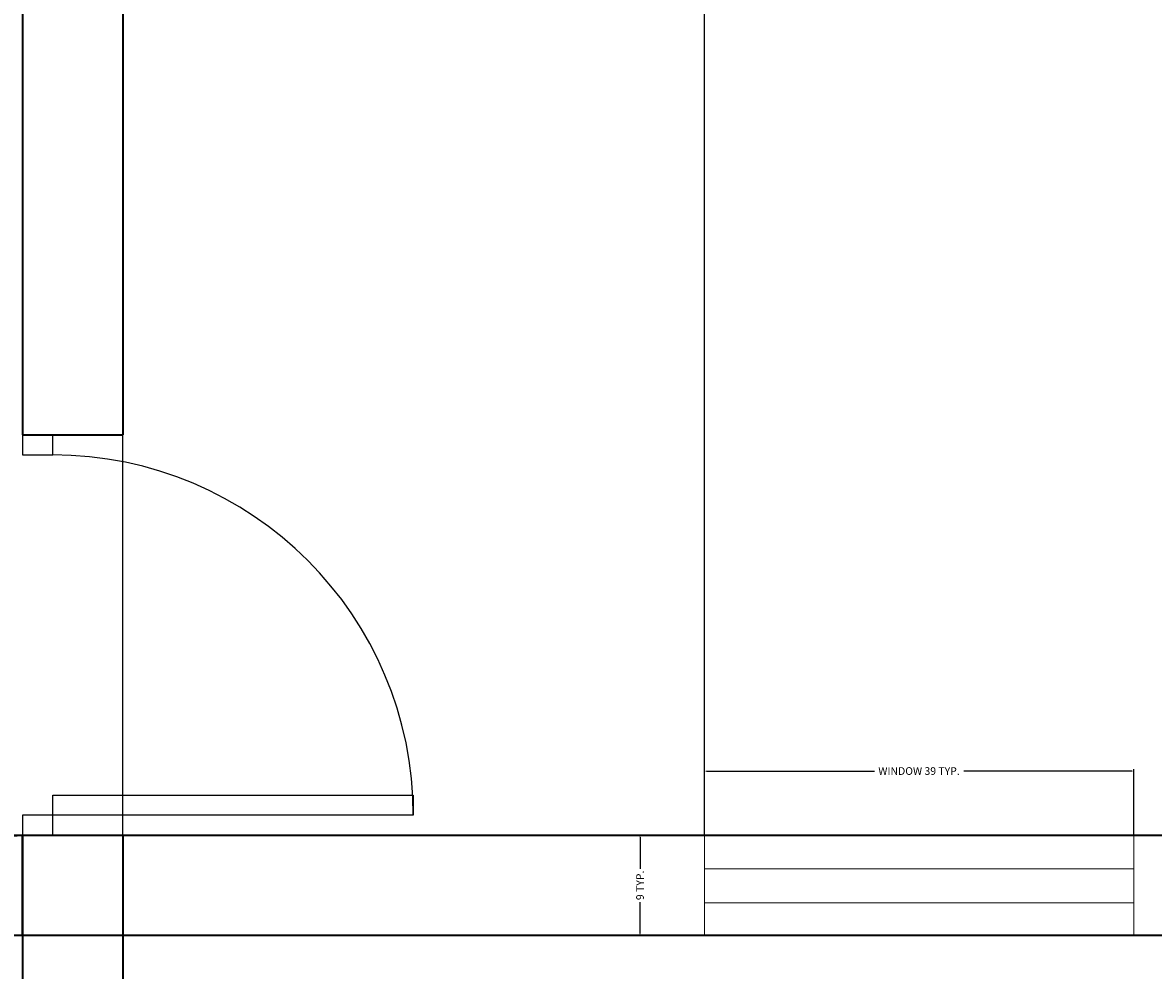
# Model space of a CAD drawing. Units: inches. Extents: x 867 to 1667, y -234 to 788.
# Tile 38 of 42: x 1395 to 1497, y 401 to 487. Entities that reach past the tile are written whole.
import ezdxf

# ---------------------------------------------------------------- set-up
doc = ezdxf.new("R2010")
doc.units = ezdxf.units.IN
doc.header["$MEASUREMENT"] = 0
for name, color, linetype, lineweight in [('A-ANNO-DIMS', 2, 'Continuous', 18), ('A-Door', 150, 'Continuous', 25), ('A-Glaz', 92, 'Continuous', 18), ('A-Wall', 7, 'Continuous', 35)]:
    doc.layers.add(name, color=color, linetype=linetype, lineweight=lineweight)
doc.layers.add('NET 01', color=8, linetype='Continuous')
doc.styles.get("Standard").update_dxf_attribs({"font": 'arial.ttf'})
doc.dimstyles.get("Standard").update_dxf_attribs({"dimtxt": 0.6875, "dimasz": 0.18, "dimexe": 0.18, "dimexo": 0.0625, "dimgap": 0.09, "dimtad": 0, "dimdec": 4, "dimzin": 0, "dimdsep": 46, "dimlunit": 4, "dimtxsty": 'Standard', "dimcen": 0.09, "dimadec": 0, "dimazin": 0, "dimtfac": 1, "dimtdec": 4, "dimtofl": 0, "dimtmove": 0, "dimatfit": 3, "dimfxl": 1, "dimtolj": 1, "dimtzin": 0, "dimarcsym": 0})

# ---------------------------------------------------------------- blocks, each defined once
blk = doc.blocks.new('A$C292B336C')
at = {"layer": 'A-Door'}
for points in [[(-0.05, 0), (-0.05, 0.9), (0, 0.9), (0, 0)], [(-0.95, 0), (-0.95, -0.075), (-0.9, -0.075), (-0.9, 0)], [(0, 0), (0, -0.075), (0.05, -0.075), (0.05, 0)]]:
    blk.add_lwpolyline(points, close=True, dxfattribs=at)
at = {"layer": 'NET 01'}
blk.add_arc((0, 0), 0.9, 90, 180, dxfattribs=at)
blk = doc.blocks.new('WIN-38_58IN')
for p, q in [((0, 9), (0, 0)), ((38.58, 0), (38.58, 9)), ((0, 6), (38.58, 6)), ((0, 2.92), (38.58, 2.92)), ((0, 0), (38.58, 0))]:
    blk.add_line(p, q)
blk = doc.blocks.new('*D13')
at = {"layer": 'A-ANNO-DIMS', "color": 0, "lineweight": -2, "transparency": 16777216}
for p, q in [((1456.15, 413.68), (1456.15, 419.58)), ((1456.33, 419.4), (1471.43, 419.4)), ((1494.56, 419.4), (1479.46, 419.4)), ((1494.74, 413.68), (1494.74, 419.58))]:
    blk.add_line(p, q, dxfattribs=at)
at = {"layer": 'A-ANNO-DIMS', "color": 0, "transparency": 16777216}
for points in [[(1456.33, 419.43), (1456.33, 419.37), (1456.15, 419.4)], [(1494.56, 419.43), (1494.56, 419.37), (1494.74, 419.4)]]:
    blk.add_solid(points, dxfattribs=at)
at = {"layer": 'Defpoints', "color": 0, "transparency": 16777216}
for p in [(1494.74, 419.4), (1456.15, 413.62), (1494.74, 413.62)]:
    blk.add_point(p, dxfattribs=at)
at = {"layer": 'A-ANNO-DIMS', "color": 0, "transparency": 16777216, "insert": (1475.44, 419.4), "char_height": 0.6875, "attachment_point": 5}
blk.add_mtext('\\A1;WINDOW 39 TYP.', dxfattribs=at)
blk = doc.blocks.new('*D14')
at = {"layer": 'A-ANNO-DIMS', "color": 0, "lineweight": -2, "transparency": 16777216}
for p, q in [((1456.09, 413.62), (1450.19, 413.62)), ((1450.37, 413.44), (1450.37, 410.61)), ((1450.37, 404.8), (1450.37, 407.62)), ((1456.09, 404.62), (1450.19, 404.62))]:
    blk.add_line(p, q, dxfattribs=at)
at = {"layer": 'A-ANNO-DIMS', "color": 0, "transparency": 16777216}
for points in [[(1450.34, 413.44), (1450.4, 413.44), (1450.37, 413.62)], [(1450.34, 404.8), (1450.4, 404.8), (1450.37, 404.62)]]:
    blk.add_solid(points, dxfattribs=at)
at = {"layer": 'Defpoints', "color": 0, "transparency": 16777216}
for p in [(1450.37, 413.62), (1456.15, 413.62), (1456.15, 404.62)]:
    blk.add_point(p, dxfattribs=at)
at = {"layer": 'A-ANNO-DIMS', "color": 0, "transparency": 16777216, "insert": (1450.37, 409.12), "char_height": 0.688, "attachment_point": 5, "rotation": 90}
blk.add_mtext('\\A1;9 TYP.', dxfattribs=at)
blk = doc.blocks.new('*D54')
at = {"layer": 'A-ANNO-DIMS', "color": 0, "lineweight": -2, "transparency": 16777216}
for p, q in [((1403.89, 413.68), (1403.89, 787.75)), ((1404.07, 787.57), (1428.77, 787.57)), ((1455.97, 787.57), (1431.27, 787.57)), ((1456.15, 413.68), (1456.15, 787.75))]:
    blk.add_line(p, q, dxfattribs=at)
at = {"layer": 'A-ANNO-DIMS', "color": 0, "transparency": 16777216}
for points in [[(1404.07, 787.6), (1404.07, 787.54), (1403.89, 787.57)], [(1455.97, 787.6), (1455.97, 787.54), (1456.15, 787.57)]]:
    blk.add_solid(points, dxfattribs=at)
at = {"layer": 'Defpoints', "color": 0, "transparency": 16777216}
for p in [(1456.15, 787.57), (1403.89, 413.62), (1456.15, 413.62)]:
    blk.add_point(p, dxfattribs=at)
at = {"layer": 'A-ANNO-DIMS', "color": 0, "transparency": 16777216, "insert": (1430.02, 787.57), "char_height": 0.688, "attachment_point": 5}
blk.add_mtext('\\A1;52.27', dxfattribs=at)

msp = doc.modelspace()

# ---------------------------------------------------------------- linework, layer by layer
at = {"layer": 'A-Wall'}
for p, q in [((1394.8866, 557.617), (1394.8866, 449.617)), ((1403.8866, 557.617), (1403.8866, 449.617)), ((1394.8866, 449.617), (1403.8866, 449.617)), ((1529.8866, 413.617), (1040.8866, 413.617)), ((1255.5362, 414.5056), (1394.8866, 404.617)), ((1394.8866, 413.617), (1256.8866, 404.617)), ((1394.8866, 413.617), (1394.8866, 136.117)), ((1394.8866, 404.617), (1394.8866, 413.617)), ((1403.8866, 413.617), (1403.8866, 136.117)), ((1559.8866, 404.617), (1040.8866, 404.617))]:
    msp.add_line(p, q, dxfattribs=at)

# ---------------------------------------------------------------- block references
at = {"layer": 'A-Door', "xscale": 36.01171521992244, "yscale": 36.01171521992244, "zscale": 36.01171521992244, "rotation": 270}
msp.add_blockref('A$C292B336C', (1397.5875, 415.4176), dxfattribs=at)
at = {"layer": 'A-Glaz'}
msp.add_blockref('WIN-38_58IN', (1456.1546, 404.617), dxfattribs=at)

# ---------------------------------------------------------------- dimensions: what is measured, and where the dimension line sits
at = {"layer": 'A-ANNO-DIMS'}
dim = msp.add_linear_dim(base=(1456.1541, 787.567), p1=(1403.8866, 413.617), p2=(1456.1541, 413.617), dimstyle='Standard', override={"dimdec": 2, "dimlfac": 1, "dimrnd": 0, "dimzin": 0, "dimdsep": 46, "dimlunit": 2}, dxfattribs=at)
dim.commit()
dim.dimension.update_dxf_attribs({"geometry": '*D54', "text_midpoint": (1430.0204, 787.567)})
dim = msp.add_linear_dim(base=(1494.7354, 419.4042), p1=(1456.1541, 413.617), p2=(1494.7354, 413.617), text='WINDOW <> TYP.', dimstyle='Standard', override={"dimdec": 0, "dimlfac": 1, "dimrnd": 0, "dimzin": 0, "dimdsep": 46, "dimlunit": 2}, dxfattribs=at)
dim.commit()
dim.dimension.update_dxf_attribs({"geometry": '*D13', "text_midpoint": (1475.4447, 419.4042)})
dim = msp.add_linear_dim(base=(1450.3669, 413.617), p1=(1456.1541, 404.617), p2=(1456.1541, 413.617), angle=90, text='<> TYP.', dimstyle='Standard', override={"dimdec": 0, "dimlfac": 1, "dimrnd": 0, "dimzin": 0, "dimdsep": 46, "dimlunit": 2}, dxfattribs=at)
dim.commit()
dim.dimension.update_dxf_attribs({"geometry": '*D14', "text_midpoint": (1450.3669, 409.117)})

doc.saveas('drawing.dxf')
